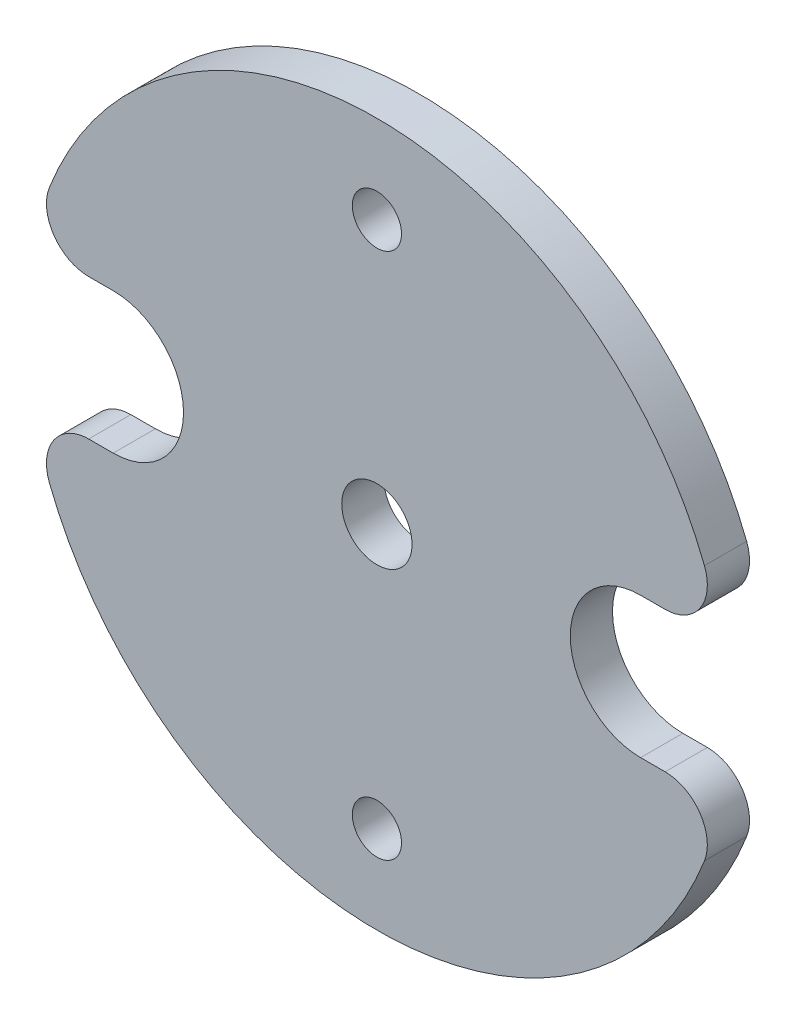
from build123d import *

# Parameters (mm, degrees)
PLATE_PROFILE_SKETCH_R   = 1.778
PLATE_PROFILE_SKETCH_R_2 = 2.54
PLATE_BODY_0_12IN_DEPTH  = 3.048
FILLETS_R0_12IN_R        = 3.048


with BuildPart() as part:
    # Plate Profile Sketch → Plate Body 0.12in (new body)
    with BuildSketch(Plane.XY):
        with BuildLine():
            Line((-19.05, 5.08), (-24.886815787, 5.08))
            ThreePointArc((-24.886815787, 5.08), (0, 25.4), (24.886815787, 5.08))
            Line((24.886815787, 5.08), (19.05, 5.08))
            ThreePointArc((19.05, 5.08), (13.97, 0), (19.05, -5.08))
            Line((19.05, -5.08), (24.886815787, -5.08))
            ThreePointArc((24.886815787, -5.08), (0, -25.4), (-24.886815787, -5.08))
            Line((-24.886815787, -5.08), (-19.05, -5.08))
            ThreePointArc((-19.05, -5.08), (-13.97, 0), (-19.05, 5.08))
        make_face()
        with Locations(Location((0, 19.05, 0), (0, 0, 180))):
            Circle(PLATE_PROFILE_SKETCH_R, mode=Mode.SUBTRACT)
        with Locations(Location((0, -19.05, 0), (0, 0, 180))):
            Circle(PLATE_PROFILE_SKETCH_R, mode=Mode.SUBTRACT)
        with Locations(Location((0, 0, 0), (0, 0, 180))):
            Circle(PLATE_PROFILE_SKETCH_R_2, mode=Mode.SUBTRACT)
    extrude(amount=PLATE_BODY_0_12IN_DEPTH)

    # Fillets R0.12in
    fillets_r0_12in_edges = [part.edges().sort_by_distance(p)[0] for p in [
        (-24.886815787, 5.08, 1.524),
        (24.886815787, 5.08, 1.524),
        (24.886815787, -5.08, 1.524),
        (-24.886815787, -5.08, 1.524),
    ]]
    fillet(fillets_r0_12in_edges, radius=FILLETS_R0_12IN_R)


solid = part.part
